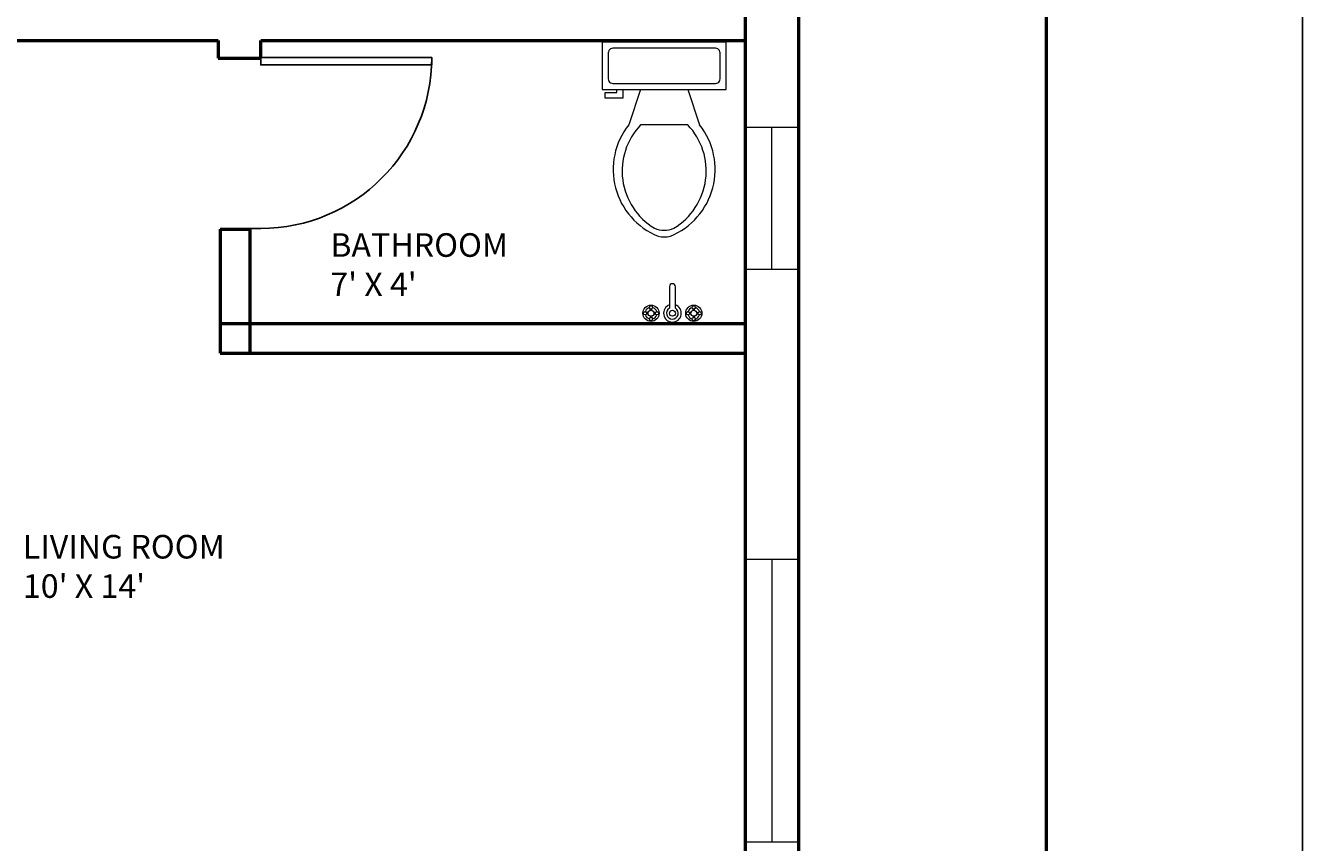
# Model space of a CAD drawing. Units: inches. Extents: x 3506 to 3958, y 1553 to 2506.
# Tile 12 of 16: x 3739 to 3957, y 2090 to 2229. Entities that reach past the tile are written whole.
import ezdxf

# ---------------------------------------------------------------- set-up
doc = ezdxf.new("R2010")
doc.units = ezdxf.units.IN
doc.header["$MEASUREMENT"] = 0
for name, color, linetype, lineweight in [('A-ANNO-DIMS', 2, 'Continuous', 18), ('A-AREA-IDEN', 7, 'Continuous', 18), ('A-WALL', 7, 'Continuous', 50), ('bathroom', 90, 'Continuous', 18), ('doors', 40, 'Continuous', 25), ('window', 30, 'Continuous', 20)]:
    doc.layers.add(name, color=color, linetype=linetype, lineweight=lineweight)
doc.layers.add('A-WALL-PATT', color=251, linetype='Continuous', lineweight=13, true_color=0x636466)
doc.styles.get("Standard").update_dxf_attribs({"font": 'arial.ttf'})
doc.dimstyles.get("Standard").update_dxf_attribs({"dimtxt": 1.18, "dimasz": 0.68, "dimexe": 0.18, "dimexo": 0.0625, "dimgap": 0.09, "dimtad": 0, "dimtih": 1, "dimtoh": 1, "dimdec": 1, "dimzin": 0, "dimdsep": 46, "dimlunit": 3, "dimtxsty": 'Standard', "dimcen": 0.09, "dimadec": 0, "dimazin": 0, "dimtfac": 1, "dimtdec": 1, "dimtofl": 0, "dimtmove": 0, "dimatfit": 3, "dimfxl": 1, "dimtolj": 1, "dimtzin": 0, "dimarcsym": 0})

# ---------------------------------------------------------------- blocks, each defined once
blk = doc.blocks.new('*U10')
for p, q in [((0, 0), (0, -6)), ((40, 0), (40, -6))]:
    blk.add_line(p, q)
blk.add_lwpolyline([(0, 0), (0, 40), (1.75, 40), (1.75, 0)], close=True)
blk.add_arc((0, 0), 40, 0, 90)
blk = doc.blocks.new('Faucet - Bathroom top')
for p, q in [((-4.107, 0.125), (-4.375, 0.125)), ((-3.75, 0.4788), (-3.75, 0.75)), ((-3.5, 0.482), (-3.5, 0.75)), ((-3.1461, 0.125), (-2.875, 0.125)), ((3.143, 0.125), (2.875, 0.125)), ((3.5, 0.4788), (3.5, 0.75)), ((3.75, 0.482), (3.75, 0.75)), ((4.1039, 0.125), (4.375, 0.125)), ((-4.1039, -0.125), (-4.375, -0.125)), ((-3.75, -0.4821), (-3.75, -0.75)), ((-3.5, -0.4789), (-3.5, -0.75)), ((-3.143, -0.125), (-2.875, -0.125)), ((-0.5, -0.8639), (-0.5, -4.5)), ((0.5, -4.5), (0.5, -0.8631)), ((3.1461, -0.125), (2.875, -0.125)), ((3.5, -0.4821), (3.5, -0.75)), ((3.75, -0.4789), (3.75, -0.75)), ((4.107, -0.125), (4.375, -0.125))]:
    blk.add_line(p, q)
for centre, radius in [((-3.625, 0), 1.375), ((-4.625, 0), 0.2795), ((-3.625, 0), 0.5), ((-3.625, 1), 0.2795), ((-2.625, 0), 0.2795), ((0, 0), 0.5), ((3.625, 0), 1.375), ((2.625, 0), 0.2795), ((3.625, 0), 0.5), ((3.625, 1), 0.2795), ((4.625, 0), 0.2795), ((-3.625, -1), 0.2795), ((3.625, -1), 0.2795)]:
    blk.add_circle(centre, radius)
for centre, radius, start, end in [((-3.625, 0), 1, 105.2407, 164.2093), ((-3.625, 0), 1, 16.44125, 74.07887), ((0, 0), 1.5, 289.6514, 250.3603), ((0, 0), 1, 300.3431, 239.7554), ((3.625, 0), 1, 106.12, 164.0884), ((3.625, 0), 1, 16.23422, 73.90469), ((-3.625, 0), 1, 196.2342, 253.9047), ((-3.625, 0), 1, 286.12, 344.0884), ((3.625, 0), 1, 196.4413, 254.0789), ((3.625, 0), 1, 285.2407, 344.2093), ((0, -4.5), 0.5, 180, 0)]:
    blk.add_arc(centre, radius, start, end)
blk = doc.blocks.new('Toilet - top')
for p, q in [((9.5, -6), (9.5, -2)), ((-10, -8.5), (-8, -8.5)), ((-10, -9.5), (-10, -8.5)), ((-8, -8.5), (-8, -8)), ((-7, -8), (-7, -9.5)), ((-4, -8), (-6, -14)), ((4, -8), (6, -14)), ((-7, -9.5), (-10, -9.5)), ((4, -14), (-4, -14))]:
    blk.add_line(p, q)
blk.add_lwpolyline([(10.5, -8), (10.5, 0), (-10.5, 0), (-10.5, -8)], close=True)
for points in [[(-9.5, -2), (-9.5, -6)], [(8.5, -1), (-8.5, -1)], [(-8.5, -7), (8.5, -7)]]:
    blk.add_lwpolyline(points)
for centre, radius, start, end in [((-8.62, -1.88), 0.884, 81.8699, 188.1301), ((8.62, -1.88), 0.884, 351.8699, 98.1301), ((-8.62, -6.12), 0.884, 171.8699, 278.1301), ((8.62, -6.12), 0.884, 261.8699, 8.1301), ((3.52, -21.58), 12.17, 141.4691, 247.9714), ((4.2, -21.82), 11.33, 136.3677, 238.9468), ((-3.52, -21.58), 12.17, 292.0284, 38.5307), ((-4.2, -21.82), 11.33, 301.053, 43.6321), ((0, -27.88), 4, 245.7318, 294.2682), ((0, -29), 4, 254.8605, 285.1395)]:
    blk.add_arc(centre, radius, start, end)
blk = doc.blocks.new('WIN-24IN-9IN-WALL')
for p, q in [((0, 0), (0, 9)), ((0, 9), (24, 9)), ((24, 9), (24, 0)), ((0, 0), (0, 4.5)), ((0, 4.5), (24, 4.5)), ((24, 0), (0, 0))]:
    blk.add_line(p, q)
blk = doc.blocks.new('WIN-48IN-9IN-WALL')
for p, q in [((0, 48), (9, 48)), ((0, 0), (0, 48)), ((0, 48), (4.5, 48)), ((4.5, 48), (4.5, 0)), ((9, 48), (9, 0)), ((9, 0), (0, 0))]:
    blk.add_line(p, q)
blk = doc.blocks.new('*D39')
at = {"layer": 'A-ANNO-DIMS', "color": 0, "lineweight": -2, "transparency": 16777216}
for p, q in [((3911.79, 2461.39), (3955.36, 2461.39)), ((3955.18, 2460.71), (3955.18, 2030.09)), ((3955.18, 1598.07), (3955.18, 2028.7)), ((3911.79, 1597.39), (3955.36, 1597.39))]:
    blk.add_line(p, q, dxfattribs=at)
at = {"layer": 'A-ANNO-DIMS', "color": 0, "transparency": 16777216}
for points in [[(3955.07, 2460.71), (3955.29, 2460.71), (3955.18, 2461.39)], [(3955.07, 1598.07), (3955.29, 1598.07), (3955.18, 1597.39)]]:
    blk.add_solid(points, dxfattribs=at)
at = {"layer": 'Defpoints', "color": 0, "transparency": 16777216}
for p in [(3911.73, 2461.39), (3955.18, 2461.39), (3911.73, 1597.39)]:
    blk.add_point(p, dxfattribs=at)
at = {"layer": 'A-ANNO-DIMS', "color": 0, "transparency": 16777216, "insert": (3955.18, 2029.39), "char_height": 1.18, "attachment_point": 5}
blk.add_mtext('\\A1;864', dxfattribs=at)
blk = doc.blocks.new('*D44')
at = {"layer": 'A-ANNO-DIMS', "color": 0, "lineweight": -2, "transparency": 16777216}
for p, q in [((3911.67, 2461.39), (3508.1, 2461.39)), ((3508.28, 2460.71), (3508.28, 2344.59)), ((3508.28, 2227.07), (3508.28, 2343.2)), ((3560.67, 2226.39), (3508.1, 2226.39))]:
    blk.add_line(p, q, dxfattribs=at)
at = {"layer": 'A-ANNO-DIMS', "color": 0, "transparency": 16777216}
for points in [[(3508.17, 2460.71), (3508.39, 2460.71), (3508.28, 2461.39)], [(3508.17, 2227.07), (3508.39, 2227.07), (3508.28, 2226.39)]]:
    blk.add_solid(points, dxfattribs=at)
at = {"layer": 'Defpoints', "color": 0, "transparency": 16777216}
for p in [(3508.28, 2461.39), (3911.73, 2461.39), (3560.73, 2226.39)]:
    blk.add_point(p, dxfattribs=at)
at = {"layer": 'A-ANNO-DIMS', "color": 0, "transparency": 16777216, "insert": (3508.28, 2343.89), "char_height": 1.18, "attachment_point": 5}
blk.add_mtext('\\A1;235', dxfattribs=at)

msp = doc.modelspace()

# ---------------------------------------------------------------- hatches: boundary and pattern name
at = {"layer": 'A-WALL-PATT'}
h = msp.add_hatch(dxfattribs=at)
h.set_pattern_fill('ANSI31', color=256)
h.paths.add_polyline_path([(3911.7302, 2461.3942), (3551.7302, 2461.3942), (3551.7302, 2152.516), (3560.7302, 2152.516), (3560.7302, 2116.516), (3551.7302, 2116.516), (3551.7302, 1920.5711), (3556.2302, 1920.5711), (3560.7302, 1920.5711), (3560.7302, 2000.3942), (3692.7302, 2000.3942), (3692.7302, 1997.3942), (3697.7302, 1997.3942), (3697.7302, 2000.3942), (3771.7302, 2000.3942), (3771.7302, 1997.3942), (3776.7302, 1997.3942), (3776.7302, 1997.7206), (3778.5802, 1997.7206), (3807.5802, 1997.7206), (3807.5802, 1996.4519), (3778.5802, 1996.4519), (3778.5802, 1997.7206), (3776.7302, 1997.7206), (3776.7302, 1997.3942), (3771.7302, 1997.3942), (3771.7302, 2000.3942), (3697.7302, 2000.3942), (3697.7302, 1997.3942), (3692.7302, 1997.3942), (3689.8302, 1997.3942), (3689.8302, 1995.8192), (3653.8302, 1995.8192), (3653.8302, 1997.3942), (3689.8302, 1997.3942), (3692.7302, 1997.3942), (3692.7302, 2000.3942), (3560.7302, 2000.3942), (3560.7302, 1920.5711), (3551.7302, 1920.5711), (3551.7302, 1884.5711), (3551.7302, 1597.3942), (3911.7302, 1597.3942)], flags=17)
h.paths.add_polyline_path([(3596.7302, 2005.3942), (3596.7302, 2057.3035, -0.38730371), (3569.1778, 2085), (3569.15, 2085), (3569.15, 2086.2688), (3598.15, 2086.2688), (3598.15, 2085), (3569.1778, 2085, 0.38730371), (3596.7302, 2057.3035), (3596.7302, 2057.3942), (3601.7302, 2057.3942), (3601.7302, 2055.3942), (3630.7302, 2055.3942), (3630.7302, 2034.3942), (3694.7302, 2034.3942), (3694.7302, 2053.3942), (3699.7302, 2053.3942), (3699.7302, 2005.3942), (3860.7302, 2005.3942), (3860.7302, 2173.3942), (3771.7302, 2173.3942), (3771.7302, 2194.3942), (3776.7302, 2194.3942), (3776.7302, 2178.3942), (3860.7302, 2178.3942), (3860.7302, 2231.3942), (3601.7302, 2231.3942), (3601.7302, 2241.426), (3596.7302, 2241.426), (3596.7302, 2231.3942), (3560.7302, 2231.3942), (3560.7302, 2315.3942), (3596.7302, 2315.3942), (3596.7302, 2312.3942), (3601.7302, 2312.3942), (3601.7302, 2315.3942), (3697.7302, 2315.3942), (3697.7302, 2413.3942), (3692.7302, 2413.3942), (3692.7302, 2320.3942), (3560.7302, 2320.3942), (3560.7302, 2452.3942), (3692.7302, 2452.3942), (3692.7302, 2449.3942), (3697.7302, 2449.3942), (3697.7302, 2452.3942), (3771.7302, 2452.3942), (3771.7302, 2449.3942), (3776.7302, 2449.3942), (3776.7302, 2452.3942), (3860.7302, 2452.3942), (3860.7302, 2437.2075), (3865.2302, 2437.2075), (3865.2302, 2413.2075), (3860.7302, 2413.2075), (3860.7302, 2367.6976), (3865.2302, 2367.6976), (3869.7302, 2367.6976), (3869.7302, 2319.6976), (3860.7302, 2319.6976), (3860.7302, 2211.6248), (3869.7302, 2211.6248), (3869.7302, 2187.6248), (3860.7302, 2187.6248), (3860.7302, 2138.4346), (3865.2302, 2138.4346), (3869.7302, 2138.4346), (3869.7302, 2090.4346), (3860.7302, 2090.4346), (3860.7302, 1985.8449), (3869.7302, 1985.8449), (3869.7302, 1961.8449), (3860.7302, 1961.8449), (3860.7302, 1897.0756), (3865.2302, 1897.0756), (3869.7302, 1897.0756), (3869.7302, 1849.0756), (3860.7302, 1849.0756), (3860.7302, 1847.8112), (3860.7302, 1779.3942), (3596.7302, 1779.3942), (3596.7302, 1831.3942), (3601.7302, 1831.3942), (3601.7302, 1828.3942), (3630.7302, 1828.3942), (3630.7302, 1808.3942), (3691.7302, 1808.3942), (3691.7302, 1815.3942), (3696.7302, 1815.3942), (3696.7302, 1779.3942), (3860.7302, 1779.3942), (3860.7302, 1947.3942), (3771.7302, 1947.3942), (3771.7302, 1968.3942), (3776.7302, 1968.3942), (3776.7302, 1952.3942), (3860.7302, 1952.3942), (3860.7302, 2005.3942)], flags=0)
h.paths.add_polyline_path([(3596.7302, 2038.8546), (3601.7302, 2038.8546), (3601.7302, 2014.8546), (3596.7302, 2014.8546)], flags=0)
h.paths.add_polyline_path([(3564.1688, 2107), (3564.1688, 2167), (3644.1688, 2167), (3644.1688, 2107)], flags=0)
h.paths.add_polyline_path([(3607.0972, 2052.0208), (3620.8472, 2052.0208, -0.41421356), (3621.9931, 2050.875), (3621.9931, 2025.6667, -0.41421356), (3620.8472, 2024.5208), (3607.0972, 2024.5208, -0.41421356), (3605.9514, 2025.6667), (3605.9514, 2050.875, -0.41421356)], flags=0)
h.paths.add_polyline_path([(3578.5688, 2115), (3565.3688, 2115), (3565.3688, 2135.8), (3578.5688, 2135.8), (3578.5688, 2138.2), (3565.3688, 2138.2), (3565.3688, 2159), (3580.5688, 2159), (3580.5688, 2153.8), (3593.7688, 2167), (3593.7688, 2151.8), (3578.5688, 2151.8)], flags=0)
h.paths.add_polyline_path([(3610.9167, 2050.875), (3620.0833, 2050.875, -0.41421356), (3620.8472, 2050.1111), (3620.8472, 2039.6076, -0.41421356), (3620.0833, 2038.8438), (3610.9167, 2038.8438, -0.41421356), (3610.1528, 2039.6076), (3610.1528, 2050.1111, -0.41421356)], flags=0)
h.paths.add_polyline_path([(3610.9167, 2037.6979), (3620.0833, 2037.6979, -0.41421356), (3620.8472, 2036.934), (3620.8472, 2026.4306, -0.41421356), (3620.0833, 2025.6667), (3610.9167, 2025.6667, -0.41421356), (3610.1528, 2026.4306), (3610.1528, 2036.934, -0.41421356)], flags=0)
h.paths.add_polyline_path([(3616.2639, 2044.7639, -1), (3614.7361, 2044.7639, -1)], flags=0)
h.paths.add_polyline_path([(3615.8819, 2044.7639, -1), (3615.1181, 2044.7639, -1)], flags=0)
h.paths.add_polyline_path([(3616.2639, 2031.7778, -1), (3614.7361, 2031.7778, -1)], flags=0)
h.paths.add_polyline_path([(3615.8819, 2031.7778, -1), (3615.1181, 2031.7778, -1)], flags=0)
h.paths.add_polyline_path([(3609.7539, 2021.7868), (3626.9586, 2021.7868), (3626.9586, 2008.8833), (3609.7539, 2008.8833)], flags=0)
h.paths.add_polyline_path([(3610.4708, 2021.07), (3621.2237, 2021.07), (3621.2237, 2009.6002), (3610.4708, 2009.6002)], flags=0)
h.paths.add_polyline_path([(3611.5461, 2019.9947), (3620.1484, 2019.9947), (3620.1484, 2010.6755), (3611.5461, 2010.6755)], flags=0)
h.paths.add_polyline_path([(3621.9405, 2021.07), (3626.2417, 2021.07), (3626.2417, 2009.6002), (3621.9405, 2009.6002)], flags=0)
h.paths.add_polyline_path([(3622.6574, 2020.3531), (3625.5248, 2020.3531), (3625.5248, 2017.4857), (3622.6574, 2017.4857)], flags=0)
h.paths.add_polyline_path([(3622.6574, 2016.7688), (3625.5248, 2016.7688), (3625.5248, 2010.317), (3622.6574, 2010.317)], flags=0)
h.paths.add_polyline_path([(3624.808, 2016.0519), (3624.808, 2013.9013), (3624.0911, 2013.9013), (3624.0911, 2013.1845), (3623.3743, 2013.1845), (3623.3743, 2013.9013), (3623.3743, 2016.0519)], flags=0)
h.paths.add_polyline_path([(3623.0158, 2012.8261), (3625.1664, 2012.8261), (3625.1664, 2012.1092), (3623.0158, 2012.1092)], flags=0)
h.paths.add_polyline_path([(3623.0158, 2011.7508), (3625.1664, 2011.7508), (3625.1664, 2011.0339), (3623.0158, 2011.0339)], flags=0)
h.paths.add_polyline_path([(3650.0591, 2031.8202), (3674.0368, 2031.8202), (3674.0368, 2012.638), (3669.2413, 2012.638), (3669.2413, 2011.8388), (3672.4383, 2011.8388), (3672.4383, 2011.0395), (3651.6576, 2011.0395), (3651.6576, 2011.8388), (3654.8546, 2011.8388), (3654.8546, 2012.638), (3650.0591, 2012.638)], flags=0)
h.paths.add_polyline_path([(3658.0517, 2024.6269, -1), (3651.6576, 2024.6269, -1)], flags=0)
h.paths.add_polyline_path([(3657.2524, 2024.6269, -1), (3652.4569, 2024.6269, -1)], flags=0)
h.paths.add_polyline_path([(3656.4532, 2024.6269, -1), (3653.2561, 2024.6269, -1)], flags=0)
h.paths.add_polyline_path([(3655.6539, 2024.6269, -1), (3654.0554, 2024.6269, -1)], flags=0)
h.paths.add_polyline_path([(3657.2524, 2017.4336, -1), (3652.4569, 2017.4336, -1)], flags=0)
h.paths.add_polyline_path([(3656.4532, 2017.4336, -1), (3653.2561, 2017.4336, -1)], flags=0)
h.paths.add_polyline_path([(3655.6539, 2017.4336, -1), (3654.0554, 2017.4336, -1)], flags=0)
h.paths.add_polyline_path([(3659.6502, 2027.8239), (3664.4457, 2027.8239), (3664.4457, 2015.0358), (3659.6502, 2015.0358)], flags=0)
h.paths.add_polyline_path([(3663.6465, 2027.0247), (3663.6465, 2015.8351), (3660.4494, 2015.8351), (3660.4494, 2027.0247)], flags=0)
h.paths.add_polyline_path([(3562.6688, 1945.5), (3642.6688, 1945.5), (3642.6688, 1885.5), (3562.6688, 1885.5)], flags=0)
h.paths.add_polyline_path([(3671.6391, 2024.6269, -1), (3666.8435, 2024.6269, -1)], flags=0)
h.paths.add_polyline_path([(3670.8398, 2024.6269, -1), (3667.6428, 2024.6269, -1)], flags=0)
h.paths.add_polyline_path([(3672.4383, 2017.4336, -1), (3666.0443, 2017.4336, -1)], flags=0)
h.paths.add_polyline_path([(3670.0405, 2024.6269, -1), (3668.442, 2024.6269, -1)], flags=0)
h.paths.add_polyline_path([(3671.6391, 2017.4336, -1), (3666.8435, 2017.4336, -1)], flags=0)
h.paths.add_polyline_path([(3670.8398, 2017.4336, -1), (3667.6428, 2017.4336, -1)], flags=0)
h.paths.add_polyline_path([(3592.2688, 1945.5), (3592.2688, 1930.3), (3577.0688, 1930.3), (3577.0688, 1893.5), (3563.8688, 1893.5), (3563.8688, 1914.3), (3577.0688, 1914.3), (3577.0688, 1916.7), (3563.8688, 1916.7), (3563.8688, 1937.5), (3579.0688, 1937.5), (3579.0688, 1932.3)], flags=0)
h.paths.add_polyline_path([(3670.0405, 2017.4336, -1), (3668.442, 2017.4336, -1)], flags=0)
h.paths.add_polyline_path([(3596.7302, 2283.3942), (3601.7302, 2283.3942), (3601.7302, 2265.426), (3599.2302, 2265.426), (3599.2302, 2241.426), (3596.7302, 2241.426), (3596.7302, 2265.426)], flags=0)
h.paths.add_polyline_path([(3596.7302, 1810.7006), (3601.7302, 1810.7006), (3601.7302, 1786.7006), (3596.7302, 1786.7006)], flags=0)
h.paths.add_polyline_path([(3560.7302, 1770.3942), (3738.7302, 1770.3942), (3738.7302, 1746.3942), (3738.7302, 1722.3942), (3748.7302, 1722.3942), (3748.7302, 1674.3942), (3560.7302, 1674.3942)], flags=0)
h.paths.add_polyline_path([(3728.7302, 1746.3942), (3728.7302, 1756.0642), (3738.7302, 1746.3942), (3728.7302, 1738.1582), (3728.7302, 1698.3942), (3591.2519, 1698.3942), (3591.2519, 1746.3942)], flags=0)
h.paths.add_polyline_path([(3771.7302, 2399.3942), (3771.7302, 2420.3942), (3776.7302, 2420.3942), (3776.7302, 2404.3942), (3776.7302, 2399.3942)], flags=0)
h.paths.add_polyline_path([(3911.7302, 2461.3942), (3551.7302, 2461.3942), (3551.7302, 2152.516), (3560.7302, 2152.516), (3560.7302, 2116.516), (3551.7302, 2116.516), (3551.7302, 1920.5711), (3560.7302, 1920.5711), (3560.7302, 2000.3942), (3692.7302, 2000.3942), (3692.7302, 1997.3942), (3697.7302, 1997.3942), (3697.7302, 2000.3942), (3771.7302, 2000.3942), (3771.7302, 1997.3942), (3776.7302, 1997.3942), (3776.7302, 1997.7206), (3778.5802, 1997.7206), (3807.5802, 1997.7206), (3807.5802, 1996.4519), (3778.5802, 1996.4519), (3778.5802, 1997.7206), (3776.7302, 1997.7206), (3776.7302, 1997.3942), (3771.7302, 1997.3942), (3771.7302, 2000.3942), (3697.7302, 2000.3942), (3697.7302, 1997.3942), (3692.7302, 1997.3942), (3689.8302, 1997.3942), (3689.8302, 1995.8192), (3653.8302, 1995.8192), (3653.8302, 1997.3942), (3689.8302, 1997.3942), (3692.7302, 1997.3942), (3692.7302, 2000.3942), (3560.7302, 2000.3942), (3560.7302, 1920.5711), (3551.7302, 1920.5711), (3551.7302, 1597.3942), (3911.7302, 1597.3942)], flags=17)

# ---------------------------------------------------------------- linework, layer by layer
at = {"layer": 'A-WALL'}
for p, q in [((3860.7302, 2249.8816), (3860.7302, 2066.516)), ((3869.7302, 2249.8816), (3869.7302, 2066.516)), ((3697.7302, 2226.3942), (3771.362, 2226.3942)), ((3771.362, 2226.3942), (3771.362, 2223.3942)), ((3778.5802, 2223.3942), (3778.5802, 2226.3942)), ((3778.5802, 2226.3942), (3860.7302, 2226.3942)), ((3771.362, 2223.3942), (3778.5802, 2223.3942)), ((3771.7302, 2194.3942), (3776.7302, 2194.3942)), ((3771.7302, 2194.3942), (3771.7302, 2173.3942)), ((3771.7302, 2194.3942), (3771.7302, 2173.3942)), ((3776.7302, 2194.3942), (3776.7302, 2173.3942)), ((3776.7302, 2194.3942), (3776.7302, 2173.3942)), ((3771.7302, 2178.3942), (3860.7302, 2178.3942)), ((3771.7302, 2173.3942), (3860.7302, 2173.3942))]:
    msp.add_line(p, q, dxfattribs=at)
msp.add_lwpolyline([(3551.7302, 2461.3942), (3911.7302, 2461.3942), (3911.7302, 1597.3942), (3551.7302, 1597.3942)], close=True, dxfattribs=at)

# ---------------------------------------------------------------- block references
at = {"layer": 'bathroom'}
msp.add_blockref('Toilet - top', (3846.9804, 2226.0805), dxfattribs=at)
at = {"layer": 'bathroom', "rotation": 180}
msp.add_blockref('Faucet - Bathroom top', (3848.375, 2180.1369), dxfattribs=at)
at = {"layer": 'doors', "xscale": 0.725, "yscale": 0.725, "zscale": 0.725, "rotation": 270}
msp.add_blockref('*U10', (3778.5802, 2223.5249), dxfattribs=at)
at = {"layer": 'window', "extrusion": (0, 0, -1), "zscale": -1, "rotation": 90.0000000000039}
msp.add_blockref('WIN-24IN-9IN-WALL', (-3860.7301, 2187.6246), dxfattribs=at)
at = {"layer": 'window'}
msp.add_blockref('WIN-48IN-9IN-WALL', (3860.73, 2090.435), dxfattribs=at)

# ---------------------------------------------------------------- texts
at = {"layer": 'A-AREA-IDEN', "attachment_point": 1}
for s, width, insert, char_height in [('4"\\P{\\H20x;BATHROOM\\P7\' X 4\'}', 25.775469, (3790.3788, 2194.039), 0.2), ("LIVING ROOM\\P10' X 14'", 79.631666, (3738.2651, 2142.5519), 4)]:
    msp.add_mtext_dynamic_manual_height_columns(s, width=width, gutter_width=1, heights=[0], dxfattribs=dict(at, insert=insert, char_height=char_height))

# ---------------------------------------------------------------- dimensions: what is measured, and where the dimension line sits
at = {"layer": 'A-ANNO-DIMS'}
for base, p1, picture, middle in [((3508.2802, 2461.3942), (3560.7302, 2226.3942), '*D44', (3508.2802, 2343.8942)), ((3955.1802, 2461.3942), (3911.7302, 1597.3942), '*D39', (3955.1802, 2029.3942))]:
    dim = msp.add_linear_dim(base=base, p1=p1, p2=(3911.7302, 2461.3942), angle=90, dimstyle='Standard', override={"dimdec": 0, "dimlfac": 1, "dimrnd": 0, "dimzin": 0, "dimdsep": 46, "dimlunit": 2}, dxfattribs=at)
    dim.commit()
    dim.dimension.update_dxf_attribs({"geometry": picture, "text_midpoint": middle})

doc.saveas('drawing.dxf')
